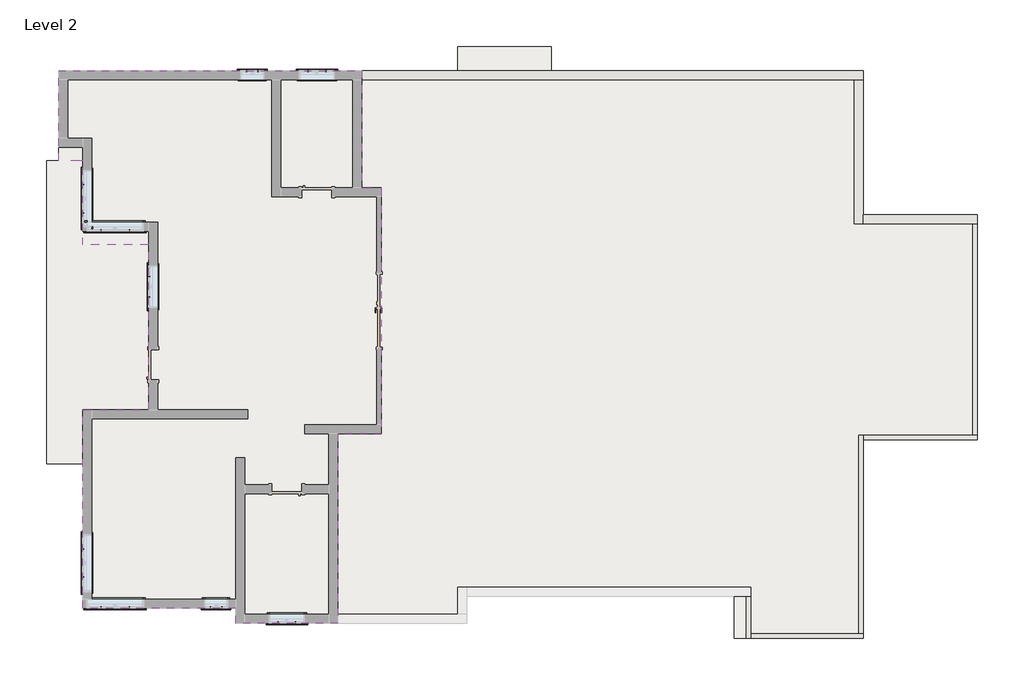
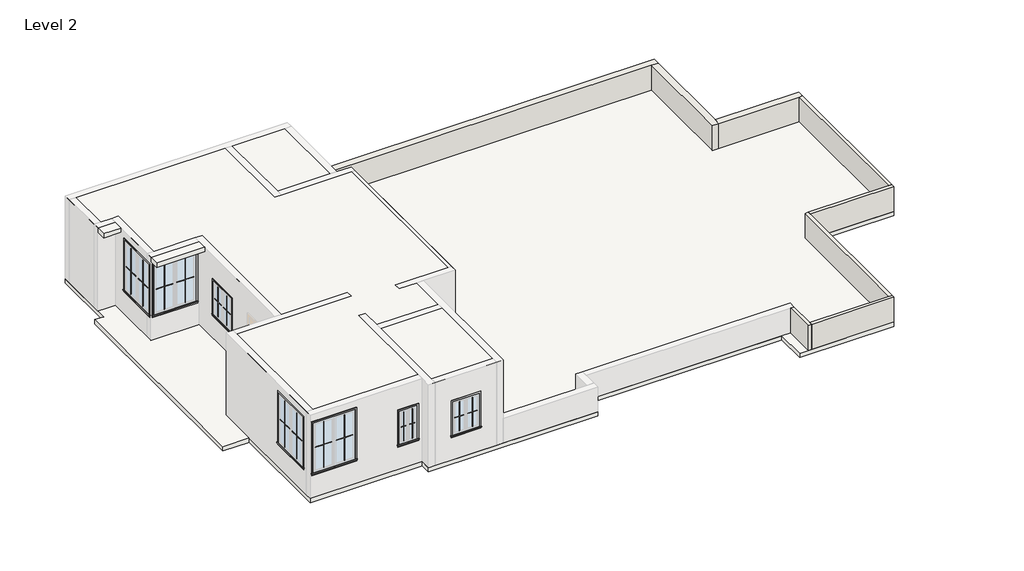
# One storey, part 2 of 2: 36 proxies, 8 walls, 2 slabs.
"""IFC4 building model written with IfcOpenShell, lengths in millimetres."""

from ifc_helpers import new_model, si_unit, frame, origin, place, context, project, spatial, polyline, outline, extrude, faceted_brep, transform, mapped, element, save
from components import muntin_pattern_2x2_muntin_pattern_2x2_ddac5204, muntin_pattern_2x2_muntin_pattern_2x2_784a3213, muntin_pattern_2x2_muntin_pattern_2x2_63e5058f, muntin_pattern_2x2_muntin_pattern_2x2_529c3de1, muntin_pattern_2x2_muntin_pattern_2x2_bff912c5, muntin_pattern_2x2_muntin_pattern_2x2_c2194282, muntin_pattern_2x2_muntin_pattern_2x2_1acec82f, muntin_pattern_2x2_muntin_pattern_2x2_43d02eee, trim_window_exterior_flat_with_sill_35723329, trim_window_exterior_flat_with_sill_245f2bb1, trim_window_exterior_flat_with_sill_e04b3088, trim_window_exterior_flat_with_sill_e4b28ec3, trim_window_interior_flat_picture_frame_e16bff95, trim_window_interior_flat_picture_frame_2b4ba637, trim_window_interior_flat_picture_frame_2a7685fe, trim_window_interior_flat_picture_frame_39ff4276

model = new_model("IFC4")

# Units and contexts
model_context = context("Model", 3, world=origin())
ifc_project = project(units=[si_unit("LENGTHUNIT", "METRE", prefix="MILLI")], contexts=[model_context])

# Site, building, storey
site = spatial("IfcSite", under=ifc_project)
building = spatial("IfcBuilding", under=site)
storey = spatial("IfcBuildingStorey", under=building, Name="Level 2", Elevation=3048.0)

# Proxies
placement = place(None, origin())
muntin_pattern_2x2_muntin_pattern_2x2_shape = muntin_pattern_2x2_muntin_pattern_2x2_ddac5204(model_context)
element("IfcBuildingElementProxy", 1, Name="Muntin Pattern_2x2 : Muntin Pattern_2x2", ObjectType="Muntin Pattern_2x2 : Muntin Pattern_2x2", at=placement, inside=storey, context=model_context, shape_type="MappedRepresentation", body=[
    mapped(muntin_pattern_2x2_muntin_pattern_2x2_shape, transform((-38531.9020004, 6033.4506148, 4032.25), x_axis=(-1.0, 0.0, 0.0), y_axis=(0.0, -1.0, 0.0), z_axis=(0.0, 0.0, 1.0))),
])
element("IfcBuildingElementProxy", 2, Name="Muntin Pattern_2x2 : Muntin Pattern_2x2", ObjectType="Muntin Pattern_2x2 : Muntin Pattern_2x2", at=placement, inside=storey, context=model_context, shape_type="MappedRepresentation", body=[
    mapped(muntin_pattern_2x2_muntin_pattern_2x2_shape, transform((-37919.1270004, 19654.2006148, 4032.25), x_axis=(1.0, 0.0, 0.0), y_axis=(0.0, 1.0, 0.0), z_axis=(0.0, 0.0, 1.0))),
])
muntin_pattern_2x2_muntin_pattern_2x2_2_shape = muntin_pattern_2x2_muntin_pattern_2x2_784a3213(model_context)
element("IfcBuildingElementProxy", 3, Name="Muntin Pattern_2x2 : Muntin Pattern_2x2", ObjectType="Muntin Pattern_2x2 : Muntin Pattern_2x2", at=placement, inside=storey, context=model_context, shape_type="MappedRepresentation", body=[
    mapped(muntin_pattern_2x2_muntin_pattern_2x2_2_shape, transform((-38833.5270004, 6033.4506148, 4032.25), x_axis=(1.0, 0.0, 0.0), y_axis=(0.0, 1.0, 0.0), z_axis=(0.0, 0.0, 1.0))),
])
element("IfcBuildingElementProxy", 4, Name="Muntin Pattern_2x2 : Muntin Pattern_2x2", ObjectType="Muntin Pattern_2x2 : Muntin Pattern_2x2", at=placement, inside=storey, context=model_context, shape_type="MappedRepresentation", body=[
    mapped(muntin_pattern_2x2_muntin_pattern_2x2_2_shape, transform((-37617.5020004, 19654.2006148, 4032.25), x_axis=(-1.0, 0.0, 0.0), y_axis=(0.0, -1.0, 0.0), z_axis=(0.0, 0.0, 1.0))),
])
muntin_pattern_2x2_muntin_pattern_2x2_3_shape = muntin_pattern_2x2_muntin_pattern_2x2_63e5058f(model_context)
element("IfcBuildingElementProxy", 5, Name="Muntin Pattern_2x2 : Muntin Pattern_2x2", ObjectType="Muntin Pattern_2x2 : Muntin Pattern_2x2", at=placement, inside=storey, context=model_context, shape_type="MappedRepresentation", body=[
    mapped(muntin_pattern_2x2_muntin_pattern_2x2_3_shape, transform((-40387.6895004, 13912.291521, 4032.25), x_axis=(0.0, 1.0, 0.0), y_axis=(-1.0, 0.0, 0.0), z_axis=(0.0, 0.0, 1.0))),
])
muntin_pattern_2x2_muntin_pattern_2x2_4_shape = muntin_pattern_2x2_muntin_pattern_2x2_529c3de1(model_context)
element("IfcBuildingElementProxy", 6, Name="Muntin Pattern_2x2 : Muntin Pattern_2x2", ObjectType="Muntin Pattern_2x2 : Muntin Pattern_2x2", at=placement, inside=storey, context=model_context, shape_type="MappedRepresentation", body=[
    mapped(muntin_pattern_2x2_muntin_pattern_2x2_4_shape, transform((-40387.6895004, 14442.516521, 4032.25), x_axis=(0.0, -1.0, 0.0), y_axis=(1.0, 0.0, 0.0), z_axis=(0.0, 0.0, 1.0))),
])
muntin_pattern_2x2_muntin_pattern_2x2_5_shape = muntin_pattern_2x2_muntin_pattern_2x2_bff912c5(model_context)
element("IfcBuildingElementProxy", 7, Name="Muntin Pattern_2x2 : Muntin Pattern_2x2", ObjectType="Muntin Pattern_2x2 : Muntin Pattern_2x2", at=placement, inside=storey, context=model_context, shape_type="MappedRepresentation", body=[
    mapped(muntin_pattern_2x2_muntin_pattern_2x2_5_shape, transform((-40887.7520004, 6033.4506148, 4032.25), x_axis=(-1.0, 0.0, 0.0), y_axis=(0.0, -1.0, 0.0), z_axis=(0.0, 0.0, 1.0))),
])
element("IfcBuildingElementProxy", 8, Name="Muntin Pattern_2x2 : Muntin Pattern_2x2", ObjectType="Muntin Pattern_2x2 : Muntin Pattern_2x2", at=placement, inside=storey, context=model_context, shape_type="MappedRepresentation", body=[
    mapped(muntin_pattern_2x2_muntin_pattern_2x2_5_shape, transform((-42064.0895004, 6806.641521, 4032.25), x_axis=(0.0, 1.0, 0.0), y_axis=(-1.0, 0.0, 0.0), z_axis=(0.0, 0.0, 1.0))),
])
element("IfcBuildingElementProxy", 9, Name="Muntin Pattern_2x2 : Muntin Pattern_2x2", ObjectType="Muntin Pattern_2x2 : Muntin Pattern_2x2", at=placement, inside=storey, context=model_context, shape_type="MappedRepresentation", body=[
    mapped(muntin_pattern_2x2_muntin_pattern_2x2_5_shape, transform((-40887.7520004, 15596.629021, 4032.25), x_axis=(-1.0, 0.0, 0.0), y_axis=(0.0, -1.0, 0.0), z_axis=(0.0, 0.0, 1.0))),
])
element("IfcBuildingElementProxy", 10, Name="Muntin Pattern_2x2 : Muntin Pattern_2x2", ObjectType="Muntin Pattern_2x2 : Muntin Pattern_2x2", at=placement, inside=storey, context=model_context, shape_type="MappedRepresentation", body=[
    mapped(muntin_pattern_2x2_muntin_pattern_2x2_5_shape, transform((-42064.0895004, 16052.241521, 4032.25), x_axis=(0.0, 1.0, 0.0), y_axis=(-1.0, 0.0, 0.0), z_axis=(0.0, 0.0, 1.0))),
])
muntin_pattern_2x2_muntin_pattern_2x2_6_shape = muntin_pattern_2x2_muntin_pattern_2x2_c2194282(model_context)
element("IfcBuildingElementProxy", 11, Name="Muntin Pattern_2x2 : Muntin Pattern_2x2", ObjectType="Muntin Pattern_2x2 : Muntin Pattern_2x2", at=placement, inside=storey, context=model_context, shape_type="MappedRepresentation", body=[
    mapped(muntin_pattern_2x2_muntin_pattern_2x2_6_shape, transform((-41608.4770004, 6033.4506148, 4032.25), x_axis=(1.0, 0.0, 0.0), y_axis=(0.0, 1.0, 0.0), z_axis=(0.0, 0.0, 1.0))),
])
element("IfcBuildingElementProxy", 12, Name="Muntin Pattern_2x2 : Muntin Pattern_2x2", ObjectType="Muntin Pattern_2x2 : Muntin Pattern_2x2", at=placement, inside=storey, context=model_context, shape_type="MappedRepresentation", body=[
    mapped(muntin_pattern_2x2_muntin_pattern_2x2_6_shape, transform((-42064.0895004, 7527.366521, 4032.25), x_axis=(0.0, -1.0, 0.0), y_axis=(1.0, 0.0, 0.0), z_axis=(0.0, 0.0, 1.0))),
])
element("IfcBuildingElementProxy", 13, Name="Muntin Pattern_2x2 : Muntin Pattern_2x2", ObjectType="Muntin Pattern_2x2 : Muntin Pattern_2x2", at=placement, inside=storey, context=model_context, shape_type="MappedRepresentation", body=[
    mapped(muntin_pattern_2x2_muntin_pattern_2x2_6_shape, transform((-41608.4770004, 15596.629021, 4032.25), x_axis=(1.0, 0.0, 0.0), y_axis=(0.0, 1.0, 0.0), z_axis=(0.0, 0.0, 1.0))),
])
element("IfcBuildingElementProxy", 14, Name="Muntin Pattern_2x2 : Muntin Pattern_2x2", ObjectType="Muntin Pattern_2x2 : Muntin Pattern_2x2", at=placement, inside=storey, context=model_context, shape_type="MappedRepresentation", body=[
    mapped(muntin_pattern_2x2_muntin_pattern_2x2_6_shape, transform((-42064.0895004, 16772.966521, 4032.25), x_axis=(0.0, -1.0, 0.0), y_axis=(1.0, 0.0, 0.0), z_axis=(0.0, 0.0, 1.0))),
])
muntin_pattern_2x2_muntin_pattern_2x2_7_shape = muntin_pattern_2x2_muntin_pattern_2x2_1acec82f(model_context)
element("IfcBuildingElementProxy", 15, Name="Muntin Pattern_2x2 : Muntin Pattern_2x2", ObjectType="Muntin Pattern_2x2 : Muntin Pattern_2x2", at=placement, inside=storey, context=model_context, shape_type="MappedRepresentation", body=[
    mapped(muntin_pattern_2x2_muntin_pattern_2x2_7_shape, transform((-36357.0270004, 19654.2006148, 4032.25), x_axis=(1.0, 0.0, 0.0), y_axis=(0.0, 1.0, 0.0), z_axis=(0.0, 0.0, 1.0))),
])
element("IfcBuildingElementProxy", 16, Name="Muntin Pattern_2x2 : Muntin Pattern_2x2", ObjectType="Muntin Pattern_2x2 : Muntin Pattern_2x2", at=placement, inside=storey, context=model_context, shape_type="MappedRepresentation", body=[
    mapped(muntin_pattern_2x2_muntin_pattern_2x2_7_shape, transform((-36665.0020004, 5652.3722085, 4032.25), x_axis=(-1.0, 0.0, 0.0), y_axis=(0.0, -1.0, 0.0), z_axis=(0.0, 0.0, 1.0))),
])
muntin_pattern_2x2_muntin_pattern_2x2_8_shape = muntin_pattern_2x2_muntin_pattern_2x2_43d02eee(model_context)
element("IfcBuildingElementProxy", 17, Name="Muntin Pattern_2x2 : Muntin Pattern_2x2", ObjectType="Muntin Pattern_2x2 : Muntin Pattern_2x2", at=placement, inside=storey, context=model_context, shape_type="MappedRepresentation", body=[
    mapped(muntin_pattern_2x2_muntin_pattern_2x2_8_shape, transform((-35903.0020004, 19654.2006148, 4032.25), x_axis=(-1.0, 0.0, 0.0), y_axis=(0.0, -1.0, 0.0), z_axis=(0.0, 0.0, 1.0))),
])
element("IfcBuildingElementProxy", 18, Name="Muntin Pattern_2x2 : Muntin Pattern_2x2", ObjectType="Muntin Pattern_2x2 : Muntin Pattern_2x2", at=placement, inside=storey, context=model_context, shape_type="MappedRepresentation", body=[
    mapped(muntin_pattern_2x2_muntin_pattern_2x2_8_shape, transform((-37119.0270004, 5652.3722085, 4032.25), x_axis=(1.0, 0.0, 0.0), y_axis=(0.0, 1.0, 0.0), z_axis=(0.0, 0.0, 1.0))),
])
trim_window_exterior_flat_with_sill_shape = trim_window_exterior_flat_with_sill_35723329(model_context)
element("IfcBuildingElementProxy", 19, Name="Trim-Window-Exterior-Flat : with Sill", ObjectType="Trim-Window-Exterior-Flat : with Sill", at=placement, inside=storey, context=model_context, shape_type="MappedRepresentation", body=[
    mapped(trim_window_exterior_flat_with_sill_shape, transform((-38682.7145004, 6023.9256148, 5181.6), x_axis=(1.0, 0.0, 0.0), y_axis=(0.0, 0.0, 1.0), z_axis=(0.0, -1.0, 0.0))),
])
element("IfcBuildingElementProxy", 20, Name="Trim-Window-Exterior-Flat : with Sill", ObjectType="Trim-Window-Exterior-Flat : with Sill", at=placement, inside=storey, context=model_context, shape_type="MappedRepresentation", body=[
    mapped(trim_window_exterior_flat_with_sill_shape, transform((-37768.3145004, 19663.7256148, 5181.6), x_axis=(-1.0, 0.0, 0.0), y_axis=(0.0, 0.0, 1.0), z_axis=(0.0, 1.0, 0.0))),
])
trim_window_exterior_flat_with_sill_2_shape = trim_window_exterior_flat_with_sill_245f2bb1(model_context)
element("IfcBuildingElementProxy", 21, Name="Trim-Window-Exterior-Flat : with Sill", ObjectType="Trim-Window-Exterior-Flat : with Sill", at=placement, inside=storey, context=model_context, shape_type="MappedRepresentation", body=[
    mapped(trim_window_exterior_flat_with_sill_2_shape, transform((-40397.2145004, 14177.404021, 5181.6), x_axis=(0.0, -1.0, 0.0), y_axis=(0.0, 0.0, 1.0), z_axis=(-1.0, 0.0, 0.0))),
])
trim_window_exterior_flat_with_sill_3_shape = trim_window_exterior_flat_with_sill_e04b3088(model_context)
element("IfcBuildingElementProxy", 22, Name="Trim-Window-Exterior-Flat : with Sill", ObjectType="Trim-Window-Exterior-Flat : with Sill", at=placement, inside=storey, context=model_context, shape_type="MappedRepresentation", body=[
    mapped(trim_window_exterior_flat_with_sill_3_shape, transform((-41248.1145004, 6023.9256148, 5791.2), x_axis=(1.0, 0.0, 0.0), y_axis=(0.0, 0.0, 1.0), z_axis=(0.0, -1.0, 0.0))),
])
element("IfcBuildingElementProxy", 23, Name="Trim-Window-Exterior-Flat : with Sill", ObjectType="Trim-Window-Exterior-Flat : with Sill", at=placement, inside=storey, context=model_context, shape_type="MappedRepresentation", body=[
    mapped(trim_window_exterior_flat_with_sill_3_shape, transform((-42073.6145004, 7167.004021, 5791.2), x_axis=(0.0, -1.0, 0.0), y_axis=(0.0, 0.0, 1.0), z_axis=(-1.0, 0.0, 0.0))),
])
element("IfcBuildingElementProxy", 24, Name="Trim-Window-Exterior-Flat : with Sill", ObjectType="Trim-Window-Exterior-Flat : with Sill", at=placement, inside=storey, context=model_context, shape_type="MappedRepresentation", body=[
    mapped(trim_window_exterior_flat_with_sill_3_shape, transform((-41248.1145004, 15587.104021, 5791.2), x_axis=(1.0, 0.0, 0.0), y_axis=(0.0, 0.0, 1.0), z_axis=(0.0, -1.0, 0.0))),
])
element("IfcBuildingElementProxy", 25, Name="Trim-Window-Exterior-Flat : with Sill", ObjectType="Trim-Window-Exterior-Flat : with Sill", at=placement, inside=storey, context=model_context, shape_type="MappedRepresentation", body=[
    mapped(trim_window_exterior_flat_with_sill_3_shape, transform((-42073.6145004, 16412.604021, 5791.2), x_axis=(0.0, -1.0, 0.0), y_axis=(0.0, 0.0, 1.0), z_axis=(-1.0, 0.0, 0.0))),
])
trim_window_exterior_flat_with_sill_4_shape = trim_window_exterior_flat_with_sill_e4b28ec3(model_context)
element("IfcBuildingElementProxy", 26, Name="Trim-Window-Exterior-Flat : with Sill", ObjectType="Trim-Window-Exterior-Flat : with Sill", at=placement, inside=storey, context=model_context, shape_type="MappedRepresentation", body=[
    mapped(trim_window_exterior_flat_with_sill_4_shape, transform((-36130.0145004, 19663.7256148, 5181.6), x_axis=(-1.0, 0.0, 0.0), y_axis=(0.0, 0.0, 1.0), z_axis=(0.0, 1.0, 0.0))),
])
element("IfcBuildingElementProxy", 27, Name="Trim-Window-Exterior-Flat : with Sill", ObjectType="Trim-Window-Exterior-Flat : with Sill", at=placement, inside=storey, context=model_context, shape_type="MappedRepresentation", body=[
    mapped(trim_window_exterior_flat_with_sill_4_shape, transform((-36892.0145004, 5642.8472085, 5181.6), x_axis=(1.0, 0.0, 0.0), y_axis=(0.0, 0.0, 1.0), z_axis=(0.0, -1.0, 0.0))),
])
trim_window_interior_flat_picture_frame_shape = trim_window_interior_flat_picture_frame_e16bff95(model_context)
element("IfcBuildingElementProxy", 28, Name="Trim-Window-Interior-Flat : Picture Frame", ObjectType="Trim-Window-Interior-Flat : Picture Frame", at=placement, inside=storey, context=model_context, shape_type="MappedRepresentation", body=[
    mapped(trim_window_interior_flat_picture_frame_shape, transform((-38682.7145004, 6252.5256148, 5181.6), x_axis=(-1.0, 0.0, 0.0), y_axis=(0.0, 0.0, 1.0), z_axis=(0.0, 1.0, 0.0))),
])
element("IfcBuildingElementProxy", 29, Name="Trim-Window-Interior-Flat : Picture Frame", ObjectType="Trim-Window-Interior-Flat : Picture Frame", at=placement, inside=storey, context=model_context, shape_type="MappedRepresentation", body=[
    mapped(trim_window_interior_flat_picture_frame_shape, transform((-37768.3145004, 19435.1256148, 5181.6), x_axis=(1.0, 0.0, 0.0), y_axis=(0.0, 0.0, 1.0), z_axis=(0.0, -1.0, 0.0))),
])
trim_window_interior_flat_picture_frame_2_shape = trim_window_interior_flat_picture_frame_2b4ba637(model_context)
element("IfcBuildingElementProxy", 30, Name="Trim-Window-Interior-Flat : Picture Frame", ObjectType="Trim-Window-Interior-Flat : Picture Frame", at=placement, inside=storey, context=model_context, shape_type="MappedRepresentation", body=[
    mapped(trim_window_interior_flat_picture_frame_2_shape, transform((-40168.6145004, 14177.404021, 5181.6), x_axis=(0.0, 1.0, 0.0), y_axis=(0.0, 0.0, 1.0), z_axis=(1.0, 0.0, 0.0))),
])
trim_window_interior_flat_picture_frame_3_shape = trim_window_interior_flat_picture_frame_2a7685fe(model_context)
element("IfcBuildingElementProxy", 31, Name="Trim-Window-Interior-Flat : Picture Frame", ObjectType="Trim-Window-Interior-Flat : Picture Frame", at=placement, inside=storey, context=model_context, shape_type="MappedRepresentation", body=[
    mapped(trim_window_interior_flat_picture_frame_3_shape, transform((-41248.1145004, 6252.5256148, 5791.2), x_axis=(-1.0, 0.0, 0.0), y_axis=(0.0, 0.0, 1.0), z_axis=(0.0, 1.0, 0.0))),
])
element("IfcBuildingElementProxy", 32, Name="Trim-Window-Interior-Flat : Picture Frame", ObjectType="Trim-Window-Interior-Flat : Picture Frame", at=placement, inside=storey, context=model_context, shape_type="MappedRepresentation", body=[
    mapped(trim_window_interior_flat_picture_frame_3_shape, transform((-41845.0145004, 7167.004021, 5791.2), x_axis=(0.0, 1.0, 0.0), y_axis=(0.0, 0.0, 1.0), z_axis=(1.0, 0.0, 0.0))),
])
element("IfcBuildingElementProxy", 33, Name="Trim-Window-Interior-Flat : Picture Frame", ObjectType="Trim-Window-Interior-Flat : Picture Frame", at=placement, inside=storey, context=model_context, shape_type="MappedRepresentation", body=[
    mapped(trim_window_interior_flat_picture_frame_3_shape, transform((-41248.1145004, 15815.704021, 5791.2), x_axis=(-1.0, 0.0, 0.0), y_axis=(0.0, 0.0, 1.0), z_axis=(0.0, 1.0, 0.0))),
])
element("IfcBuildingElementProxy", 34, Name="Trim-Window-Interior-Flat : Picture Frame", ObjectType="Trim-Window-Interior-Flat : Picture Frame", at=placement, inside=storey, context=model_context, shape_type="MappedRepresentation", body=[
    mapped(trim_window_interior_flat_picture_frame_3_shape, transform((-41845.0145004, 16412.604021, 5791.2), x_axis=(0.0, 1.0, 0.0), y_axis=(0.0, 0.0, 1.0), z_axis=(1.0, 0.0, 0.0))),
])
trim_window_interior_flat_picture_frame_4_shape = trim_window_interior_flat_picture_frame_39ff4276(model_context)
element("IfcBuildingElementProxy", 35, Name="Trim-Window-Interior-Flat : Picture Frame", ObjectType="Trim-Window-Interior-Flat : Picture Frame", at=placement, inside=storey, context=model_context, shape_type="MappedRepresentation", body=[
    mapped(trim_window_interior_flat_picture_frame_4_shape, transform((-36130.0145004, 19435.1256148, 5181.6), x_axis=(1.0, 0.0, 0.0), y_axis=(0.0, 0.0, 1.0), z_axis=(0.0, -1.0, 0.0))),
])
element("IfcBuildingElementProxy", 36, Name="Trim-Window-Interior-Flat : Picture Frame", ObjectType="Trim-Window-Interior-Flat : Picture Frame", at=placement, inside=storey, context=model_context, shape_type="MappedRepresentation", body=[
    mapped(trim_window_interior_flat_picture_frame_4_shape, transform((-36892.0145004, 5871.4472085, 5181.6), x_axis=(-1.0, 0.0, 0.0), y_axis=(0.0, 0.0, 1.0), z_axis=(0.0, 1.0, 0.0))),
])

# Slabs
element("IfcSlab", 37, ObjectType="slab 6\"", at=placement, inside=storey, context=model_context, shape_type="SweptSolid", body=[
    extrude(outline(polyline([(-32548.6145004, 19663.7256148), (-32548.6145004, 20273.3256148), (-30186.4145004, 20273.3256148), (-30186.4145004, 19663.7256148), (-22261.6145004, 19663.7256148), (-22261.6145004, 16006.1256148), (-19366.0145004, 16006.1256148), (-19366.0145004, 10291.1256148), (-22261.6145004, 10291.1256148), (-22261.6145004, 5261.5453879), (-25538.2145004, 5261.5453879), (-25538.2145004, 6328.7256148), (-32320.0145004, 6328.7256148), (-32320.0145004, 5642.8472085), (-38187.4145004, 5642.8472085), (-38187.4145004, 6023.9256148), (-42073.6145004, 6023.9256148), (-42073.6145004, 9681.5256148), (-42988.0145004, 9681.5256148), (-42988.0145004, 17377.7256148), (-42683.2145004, 17377.7256148), (-42683.2145004, 19663.7256148), (-32548.6145004, 19663.7256148)])), frame((0.0, 0.0, 2895.6), z_axis=(0.0, 0.0, 1.0), x_axis=(1.0, 0.0, 0.0)), (0.0, 0.0, 1.0), 152.4),
])
element("IfcSlab", 38, ObjectType="slab 6\"", at=placement, inside=storey, context=model_context, shape_type="SweptSolid", body=[
    extrude(outline(polyline([(-34986.3753088, 19663.7504636), (-34986.3753088, 16691.9504636), (-34491.0753088, 16691.9504636), (-34491.0753088, 16234.7504636), (-34491.0753088, 10443.5504636), (-35595.9753088, 10443.5504636), (-35595.9753088, 5642.8720573), (-38186.7753088, 5642.8720573), (-38186.7753088, 6023.9504636), (-42072.9753088, 6023.9504636), (-42072.9753088, 11053.1504636), (-40396.0832488, 11053.1504636), (-40396.0832488, 15244.1504636), (-42072.9753088, 15244.1504636), (-42072.9753088, 17377.7504636), (-42682.5753088, 17377.7504636), (-42682.5753088, 19663.7504636), (-34986.3753088, 19663.7504636)])), frame((0.0, 0.0, 5943.6), z_axis=(0.0, 0.0, 1.0), x_axis=(1.0, 0.0, 0.0)), (0.0, 0.0, 1.0), 152.4),
])

# Walls
element("IfcWall", 39, ObjectType="wall 4.5", at=placement, inside=storey, context=model_context, shape_type="Brep", body=[
    faceted_brep([(-25233.4145004, 6328.7256148, 3048.0), (-25233.4145004, 5261.9256148, 3048.0), (-25233.4145004, 5261.9256148, 3962.4), (-25233.4145004, 6328.7256148, 3962.4), (-25119.1145004, 6328.7256148, 3048.0), (-25119.1145004, 6328.7256148, 3962.4), (-25119.1145004, 5376.2256148, 3962.4), (-25119.1145004, 5261.9256148, 3962.4), (-25119.1145004, 5261.9256148, 3048.0), (-25119.1145004, 5376.2256148, 3048.0)], [[[0, 1, 2, 3]], [[4, 5, 6, 7, 8, 9]], [[1, 0, 4, 9, 8]], [[3, 2, 7, 6, 5]], [[0, 3, 5, 4]], [[2, 1, 8, 7]]]),
])
element("IfcWall", 40, ObjectType="wall 4.5", at=placement, inside=storey, context=model_context, shape_type="Brep", body=[
    faceted_brep([(-25119.1145004, 5261.9256148, 3048.0), (-22261.6145004, 5261.9256148, 3048.0), (-22261.6145004, 5261.9256148, 3962.4), (-25119.1145004, 5261.9256148, 3962.4), (-25119.1145004, 5376.2256148, 3048.0), (-25119.1145004, 5376.2256148, 3962.4), (-22375.9145004, 5376.2256148, 3962.4), (-22261.6145004, 5376.2256148, 3962.4), (-22261.6145004, 5376.2256148, 3048.0), (-22375.9145004, 5376.2256148, 3048.0)], [[[0, 1, 2, 3]], [[4, 5, 6, 7, 8, 9]], [[1, 0, 4, 9, 8]], [[3, 2, 7, 6, 5]], [[0, 3, 5, 4]], [[2, 1, 8, 7]]]),
])
element("IfcWall", 41, ObjectType="wall 4.5", at=placement, inside=storey, context=model_context, shape_type="Brep", body=[
    faceted_brep([(-22261.6145004, 5376.2256148, 3048.0), (-22261.6145004, 10291.1256148, 3048.0), (-22261.6145004, 10405.4256148, 3048.0), (-22261.6145004, 10405.4256148, 3962.4), (-22261.6145004, 10291.1256148, 3962.4), (-22261.6145004, 5376.2256148, 3962.4), (-22375.9145004, 5376.2256148, 3048.0), (-22375.9145004, 5376.2256148, 3962.4), (-22375.9145004, 10405.4256148, 3962.4), (-22375.9145004, 10405.4256148, 3048.0)], [[[0, 1, 2, 3, 4, 5]], [[6, 7, 8, 9]], [[2, 1, 0, 6, 9]], [[5, 4, 3, 8, 7]], [[0, 5, 7, 6]], [[3, 2, 9, 8]]]),
])
element("IfcWall", 42, ObjectType="wall 4.5", at=placement, inside=storey, context=model_context, shape_type="Brep", body=[
    faceted_brep([(-22261.6145004, 10291.1256148, 3048.0), (-19366.0145004, 10291.1256148, 3048.0), (-19366.0145004, 10291.1256148, 3962.4), (-22261.6145004, 10291.1256148, 3962.4), (-22261.6145004, 10405.4256148, 3048.0), (-22261.6145004, 10405.4256148, 3962.4), (-19480.3145004, 10405.4256148, 3962.4), (-19366.0145004, 10405.4256148, 3962.4), (-19366.0145004, 10405.4256148, 3048.0), (-19480.3145004, 10405.4256148, 3048.0)], [[[0, 1, 2, 3]], [[4, 5, 6, 7, 8, 9]], [[1, 0, 4, 9, 8]], [[3, 2, 7, 6, 5]], [[0, 3, 5, 4]], [[2, 1, 8, 7]]]),
])
element("IfcWall", 43, ObjectType="wall 4.5", at=placement, inside=storey, context=model_context, shape_type="SweptSolid", body=[
    extrude(outline(polyline([(-19366.0145004, 15777.5256148), (-19366.0145004, 10405.4256148), (-19480.3145004, 10405.4256148), (-19480.3145004, 15777.5256148), (-19366.0145004, 15777.5256148)])), frame((0.0, 0.0, 3048.0), z_axis=(0.0, 0.0, 1.0), x_axis=(1.0, 0.0, 0.0)), (0.0, 0.0, 1.0), 914.4),
])
element("IfcWall", 44, ObjectType="wall 9\"", at=placement, inside=storey, context=model_context, shape_type="Brep", body=[
    faceted_brep([(-34987.0145004, 19435.1256148, 3048.0), (-22490.2145004, 19435.1256148, 3048.0), (-22261.6145004, 19435.1256148, 3048.0), (-22261.6145004, 19435.1256148, 3962.4), (-22490.2145004, 19435.1256148, 3962.4), (-34987.0145004, 19435.1256148, 3962.4), (-34987.0145004, 19663.7256148, 3048.0), (-34987.0145004, 19663.7256148, 3962.4), (-22261.6145004, 19663.7256148, 3962.4), (-22261.6145004, 19663.7256148, 3048.0)], [[[0, 1, 2, 3, 4, 5]], [[6, 7, 8, 9]], [[2, 1, 0, 6, 9]], [[5, 4, 3, 8, 7]], [[3, 2, 9, 8]], [[0, 5, 7, 6]]]),
])
element("IfcWall", 45, ObjectType="wall 9\"", at=placement, inside=storey, context=model_context, shape_type="Brep", body=[
    faceted_brep([(-22490.2145004, 19435.1256148, 3048.0), (-22490.2145004, 15777.5256148, 3048.0), (-22490.2145004, 15777.5256148, 3962.4), (-22490.2145004, 19435.1256148, 3962.4), (-22261.6145004, 19435.1256148, 3048.0), (-22261.6145004, 19435.1256148, 3962.4), (-22261.6145004, 16006.1256148, 3962.4), (-22261.6145004, 15777.5256148, 3962.4), (-22261.6145004, 15777.5256148, 3048.0), (-22261.6145004, 16006.1256148, 3048.0)], [[[0, 1, 2, 3]], [[4, 5, 6, 7, 8, 9]], [[1, 0, 4, 9, 8]], [[3, 2, 7, 6, 5]], [[0, 3, 5, 4]], [[2, 1, 8, 7]]]),
])
element("IfcWall", 46, ObjectType="wall 9\"", at=placement, inside=storey, context=model_context, shape_type="Brep", body=[
    faceted_brep([(-22261.6145004, 15777.5256148, 3048.0), (-19480.3145004, 15777.5256148, 3048.0), (-19366.0145004, 15777.5256148, 3048.0), (-19366.0145004, 15777.5256148, 3962.4), (-19480.3145004, 15777.5256148, 3962.4), (-22261.6145004, 15777.5256148, 3962.4), (-22261.6145004, 16006.1256148, 3048.0), (-22261.6145004, 16006.1256148, 3962.4), (-19366.0145004, 16006.1256148, 3962.4), (-19366.0145004, 16006.1256148, 3048.0)], [[[0, 1, 2, 3, 4, 5]], [[6, 7, 8, 9]], [[2, 1, 0, 6, 9]], [[5, 4, 3, 8, 7]], [[0, 5, 7, 6]], [[3, 2, 9, 8]]]),
])

save(model, "model.ifc")

# Revit data of these elements
# Type "Muntin Pattern_2x2 : Muntin Pattern_2x2"
#   Width [instance default] = 4' - 0"
#   Thickness = 0' - 0 1/2"
#   Height [instance default] = 4' - 0"
#   Distance = 0' - 0 3/4"
#   Interior Material [instance default] = none
#   Exterior Material [instance default] = none
#   Default Elevation = 0
# Type "Trim-Window-Exterior-Flat : with Sill"
#   Trim Width = 0' - 2 1/4"
#   Trim Thickness_Picture Frame = 0' - 1 1/4"
#   Trim Thickness_with Sill = 0' - 0 3/4"
#   Sill Thickness = 0' - 1 1/4"
#   Opening Width [instance default] = 2' - 0"
#   Opening Height [instance default] = 3' - 0"
#   Default Elevation = 4' - 0"
#   Sill = yes
#   Picture Frame = no
#   Trim Material [instance default] = none
# Type "Trim-Window-Interior-Flat : Picture Frame"
#   Trim Thickness_Picture Frame = 0' - 1 1/4"
#   Trim Width = 0' - 2 1/4"
#   Trim Thickness_with Sill = 0' - 0 3/4"
#   Sill Thickness = 0' - 1 1/4"
#   Opening Width [instance default] = 2' - 0"
#   Opening Height [instance default] = 3' - 0"
#   Default Elevation = 4' - 0"
#   Sill = no
#   Picture Frame = yes
#   Trim Material [instance default] = none
# Type "slab 6\""
#   Assembly Code = "B1010"
#   Function = 0
#   Layers, outside or top first: 0' - 6" no material (function 1)
# Type "wall 4.5"
#   Assembly Code = "B2010"
#   Layers, outside or top first: 0' - 4 1/2" no material (function 1)
# Type "wall 9\""
#   Assembly Code = "B2010"
#   Layers, outside or top first: 0' - 9" no material (function 1)
# Elements 1, 2, 3, 4 (IfcBuildingElementProxy, "Muntin Pattern_2x2 : Muntin Pattern_2x2")
#   Width = 0' - 6 5/8"
#   Height = 3' - 6 1/2"
#   Interior Material = Wood - Stained
#   Exterior Material = Clad - White
#   Phase Created = New Construction
#   Materials on its faces: "Clad - White", "Wood - Stained"
# Elements 5, 6 (IfcBuildingElementProxy, "Muntin Pattern_2x2 : Muntin Pattern_2x2")
#   Width = 1' - 3 5/8"
#   Height = 3' - 6 1/2"
#   Interior Material = Wood - Stained
#   Exterior Material = Clad - White
#   Phase Created = New Construction
#   Materials on its faces: "Clad - White", "Wood - Stained"
# Elements 7, 8, 9, 10, 11, 12, 13, 14 (IfcBuildingElementProxy, "Muntin Pattern_2x2 : Muntin Pattern_2x2")
#   Width = 1' - 11 1/8"
#   Height = 5' - 6 1/2"
#   Interior Material = Wood - Stained
#   Exterior Material = Clad - White
#   Phase Created = New Construction
#   Materials on its faces: "Clad - White", "Wood - Stained"
# Elements 15, 16, 17, 18 (IfcBuildingElementProxy, "Muntin Pattern_2x2 : Muntin Pattern_2x2")
#   Width = 1' - 0 5/8"
#   Height = 3' - 6 1/2"
#   Interior Material = Wood - Stained
#   Exterior Material = Clad - White
#   Phase Created = New Construction
#   Materials on its faces: "Clad - White", "Wood - Stained"
# Elements 19, 20 (IfcBuildingElementProxy, "Trim-Window-Exterior-Flat : with Sill")
#   Opening Width = 2' - 0"
#   Opening Height = 4' - 0"
#   Trim Material = Clad - White
#   Phase Created = New Construction
#   Materials on its faces: "Clad - White"
# Element 21 (IfcBuildingElementProxy, "Trim-Window-Exterior-Flat : with Sill")
#   Opening Width = 3' - 6"
#   Opening Height = 4' - 0"
#   Trim Material = Clad - White
#   Phase Created = New Construction
#   Materials on its faces: "Clad - White"
# Elements 22, 23, 24, 25 (IfcBuildingElementProxy, "Trim-Window-Exterior-Flat : with Sill")
#   Opening Width = 4' - 9"
#   Opening Height = 6' - 0"
#   Trim Material = Clad - White
#   Phase Created = New Construction
#   Materials on its faces: "Clad - White"
# Elements 26, 27 (IfcBuildingElementProxy, "Trim-Window-Exterior-Flat : with Sill")
#   Opening Width = 3' - 0"
#   Opening Height = 4' - 0"
#   Trim Material = Clad - White
#   Phase Created = New Construction
#   Materials on its faces: "Clad - White"
# Elements 28, 29 (IfcBuildingElementProxy, "Trim-Window-Interior-Flat : Picture Frame")
#   Opening Width = 2' - 0"
#   Opening Height = 4' - 0"
#   Trim Material = Wood - Stained
#   Phase Created = New Construction
#   Materials on its faces: "Wood - Stained"
# Element 30 (IfcBuildingElementProxy, "Trim-Window-Interior-Flat : Picture Frame")
#   Opening Width = 3' - 6"
#   Opening Height = 4' - 0"
#   Trim Material = Wood - Stained
#   Phase Created = New Construction
#   Materials on its faces: "Wood - Stained"
# Elements 31, 32, 33, 34 (IfcBuildingElementProxy, "Trim-Window-Interior-Flat : Picture Frame")
#   Opening Width = 4' - 9"
#   Opening Height = 6' - 0"
#   Trim Material = Wood - Stained
#   Phase Created = New Construction
#   Materials on its faces: "Wood - Stained"
# Elements 35, 36 (IfcBuildingElementProxy, "Trim-Window-Interior-Flat : Picture Frame")
#   Opening Width = 3' - 0"
#   Opening Height = 4' - 0"
#   Trim Material = Wood - Stained
#   Phase Created = New Construction
#   Materials on its faces: "Wood - Stained"
# Element 37 (IfcSlab, "slab 6\"")
#   Height Offset From Level = 0' - 0"
#   Phase Created = New Construction
#   Materials on its faces: "Default Floor"
# Element 38 (IfcSlab, "slab 6\"")
#   Height Offset From Level = 10' - 0"
#   Phase Created = New Construction
#   Materials on its faces: "Default Floor"
# Elements 39, 40, 41, 42, 43 (IfcWall, "wall 4.5")
#   Top Offset = 0' - 0"
#   Base Offset = 0' - 0"
#   wall height = 3' - 0"
#   Phase Created = New Construction
#   Base Constraint = Level 2
#   Top Constraint = Level 8
#   Materials on its faces: "Default Wall"
# Elements 44, 45, 46 (IfcWall, "wall 9\"")
#   Top Offset = 0' - 0"
#   Base Offset = 0' - 0"
#   wall height = 3' - 0"
#   Phase Created = New Construction
#   Base Constraint = Level 2
#   Top Constraint = Level 8
#   Materials on its faces: "Default Wall"
# Materials
#   "Clad - White": class "Wood", colour RGB 242 242 238, transparency 0, Cost = 0
#   "Wood - Stained": class "Wood", colour RGB 224 178 126, transparency 0, Cost = 0
#   "Default Floor": colour RGB 128 128 128, transparency 0, Cost = 0
#   "Default Wall": colour RGB 128 128 128, transparency 0, Cost = 0
